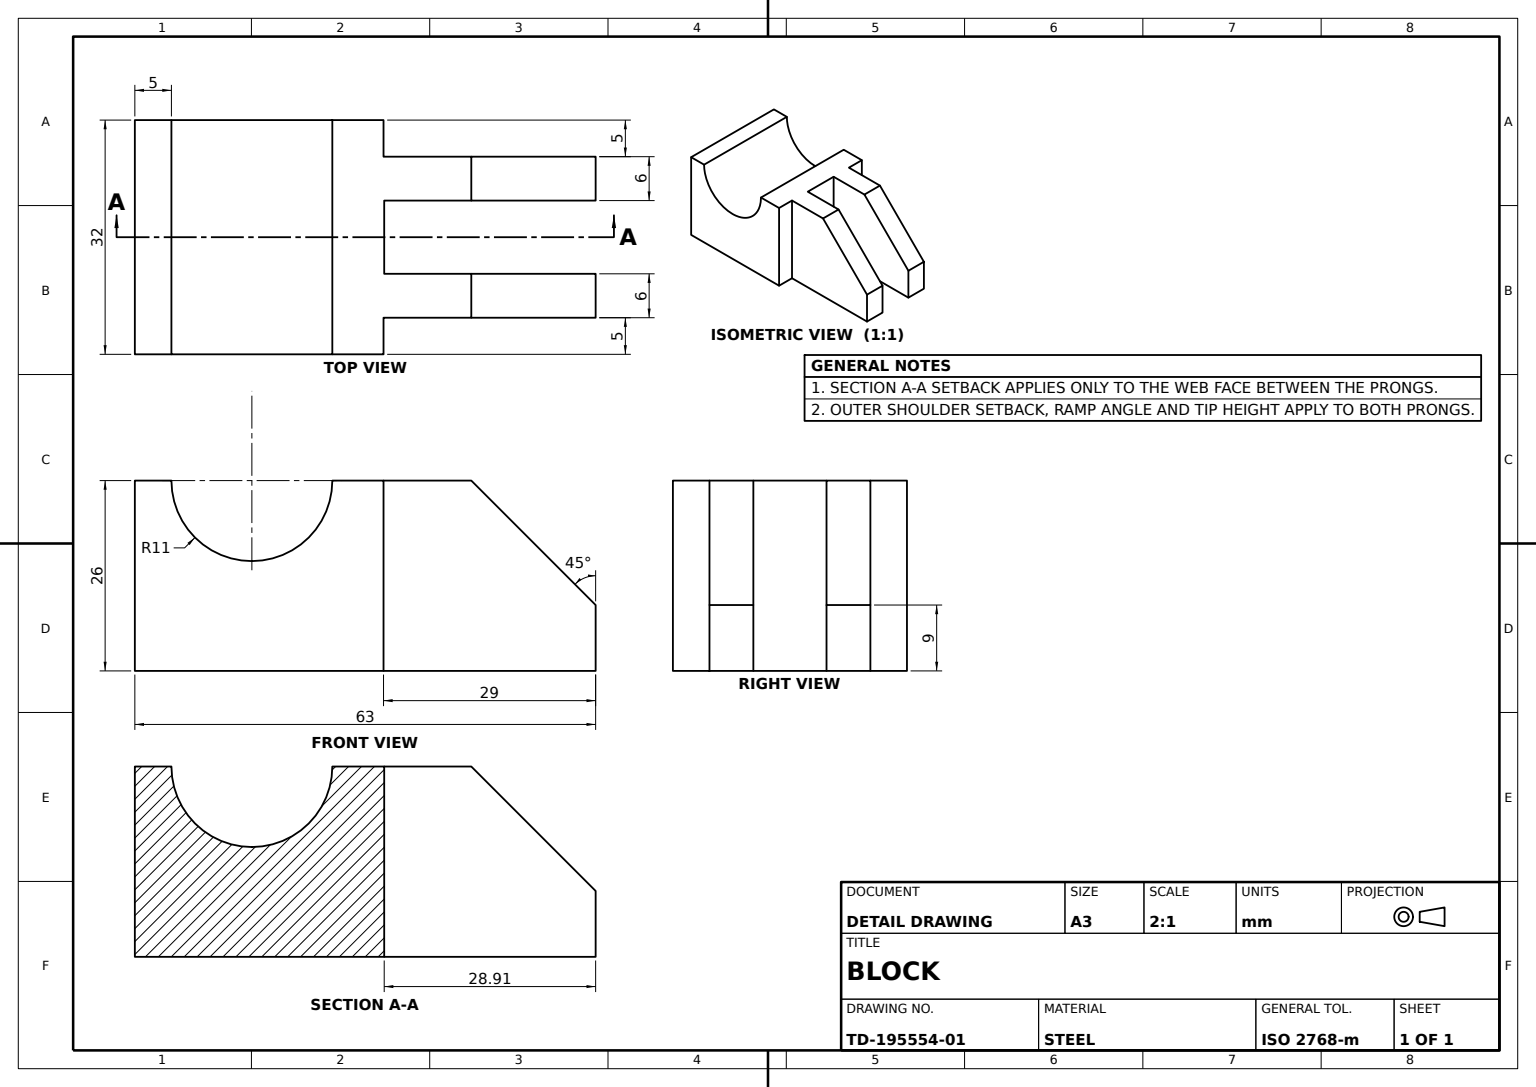
from build123d import *

# Parameters (mm, degrees)
BASE_BLOCK_PROFILE_63X32_W  = 63
BASE_BLOCK_PROFILE_63X32_H  = 32
BASE_BLOCK_63X32X26_DEPTH   = 26
BORE_SLOT_CUT_DEPTH         = 32
RECTANGULAR_SLOT_17X9_DEPTH = 32
SIDE_STEP_PROFILE_W         = 29
SIDE_STEP_PROFILE_H         = 5
SIDE_STEP_CUT_DEPTH         = 44.866274061
SIDE_GROOVE_CUT_DEPTH       = 44.866274061


with BuildPart() as part:
    # Base Block Profile 63x32 → Base Block 63x32x26 (new body)
    with BuildSketch(Plane.XY):
        Rectangle(BASE_BLOCK_PROFILE_63X32_W, BASE_BLOCK_PROFILE_63X32_H)
    extrude(amount=BASE_BLOCK_63X32X26_DEPTH)

    # Bore Slot Profile → Bore Slot Cut (cut)
    with BuildSketch(Plane.XZ.offset(16)):
        with BuildLine():
            ThreePointArc((4.5, 26), (15.5, 15), (26.5, 26))
            Line((26.5, 26), (4.5, 26))
        make_face()
    extrude(amount=-BORE_SLOT_CUT_DEPTH, mode=Mode.SUBTRACT)

    # Rectangular Slot Profile 17x9 → Rectangular Slot 17x9 (cut)
    with BuildSketch(Plane(origin=(0, -16, 0), x_dir=(-1, 0, 0), z_dir=(0, -1, 0))):
        Polygon((31.5, -9), (14.5, -26), (31.5, -26), align=None)
    extrude(amount=-RECTANGULAR_SLOT_17X9_DEPTH, mode=Mode.SUBTRACT)

    # Side Step Profile → Side Step Cut (cut, through all)
    with BuildSketch(Plane(origin=(0, 0, 0), x_dir=(-1, 0, 0), z_dir=(0, 0, -1))):
        with Locations((17, 13.5)):
            Rectangle(SIDE_STEP_PROFILE_W, SIDE_STEP_PROFILE_H)
        with Locations((17, -13.5)):
            Rectangle(SIDE_STEP_PROFILE_W, SIDE_STEP_PROFILE_H)
    extrude(amount=-SIDE_STEP_CUT_DEPTH, mode=Mode.SUBTRACT)

    # Side Groove Profile → Side Groove Cut (cut, through all)
    with BuildSketch(Plane(origin=(0, 0, 0), x_dir=(-1, 0, 0), z_dir=(0, 0, -1))):
        Polygon((31.5, -5.002946395), (31.5, 0), (31.5, 5), (2.592435859, 5), (2.592435859, -5.002946395), align=None)
    extrude(amount=-SIDE_GROOVE_CUT_DEPTH, mode=Mode.SUBTRACT)


solid = part.part
